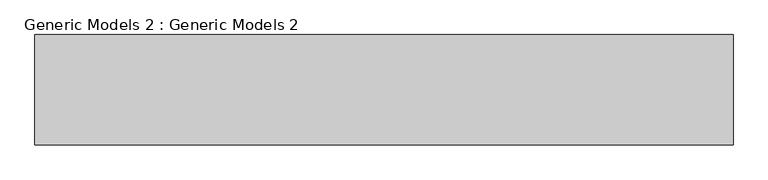
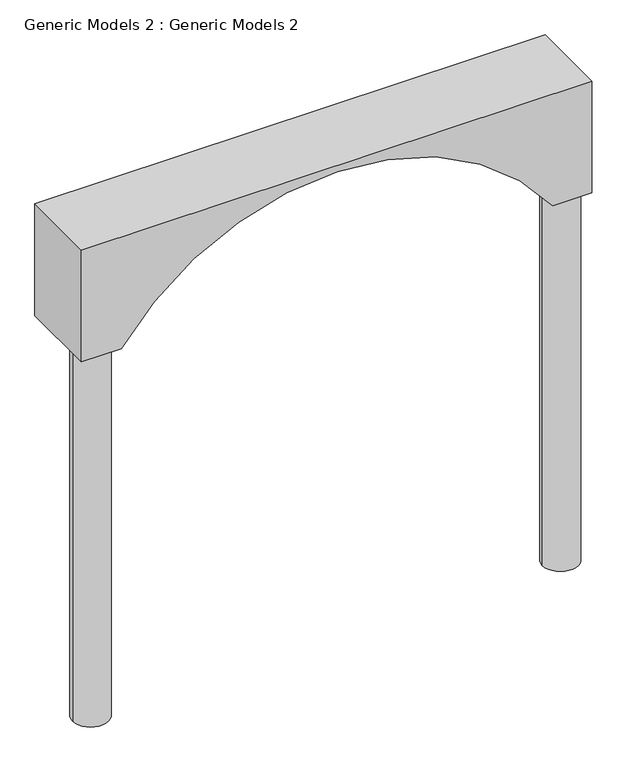
"""IFC4 building model written with IfcOpenShell, lengths in millimetres: proxy geometry, Generic Models 2 : Generic Models 2."""

from ifc_helpers import new_model, si_unit, point, frame, frame_2d, origin, origin_with_axes, place, context, project, spatial, polyline, circle_curve, trimmed, segment, composite_curve, outline, extrude, source, transform, mapped, element, save


def generic_models_2_generic_models_2_701112c8(model_context):
    return source(origin(), model_context, "Body", "SweptSolid", [
        extrude(outline(composite_curve([segment(trimmed(circle_curve(frame_2d((-14185.0310619, 3684.6465918)), 101.6), [point((-14286.6310619, 3684.6465918))], [point((-14083.4310619, 3684.6465918))], False, "CARTESIAN"), True, "CONTINUOUS"), segment(trimmed(circle_curve(frame_2d((-14185.0310619, 3684.6465918)), 101.6), [point((-14083.4310619, 3684.6465918))], [point((-14286.6310619, 3684.6465918))], False, "CARTESIAN"), True, "CONTINUOUS")], self_intersect=False)), origin_with_axes(), (0.0, 0.0, 1.0), 2226.4463041),
        extrude(outline(composite_curve([segment(trimmed(circle_curve(frame_2d((-11520.4016034, 3684.6465918)), 101.6), [point((-11418.8016034, 3684.6465918))], [point((-11622.0016034, 3684.6465918))], False, "CARTESIAN"), True, "CONTINUOUS"), segment(trimmed(circle_curve(frame_2d((-11520.4016034, 3684.6465918)), 101.6), [point((-11622.0016034, 3684.6465918))], [point((-11418.8016034, 3684.6465918))], False, "CARTESIAN"), True, "CONTINUOUS")], self_intersect=False)), origin_with_axes(), (0.0, 0.0, 1.0), 2226.4463041),
        extrude(outline(composite_curve([segment(polyline([(2226.4463041, -11627.5105536), (2226.4463041, -11405.0590017), (2895.6, -11405.0590017), (2895.6, -14300.3736637), (2226.4463041, -14300.3736637), (2226.4463041, -14074.0083114)]), True, "CONTINUOUS"), segment(trimmed(circle_curve(frame_2d((1360.7303343, -12850.7594325)), 1498.6), [point((2226.4463041, -14074.0083114))], [point((2226.4463041, -11627.5105536))], True, "CARTESIAN"), True, "CONTINUOUS")], self_intersect=False)), frame((0.0, 3574.2170165, 0.0), z_axis=(0.0, 1.0, 0.0), x_axis=(0.0, 0.0, 1.0)), (0.0, 0.0, 1.0), 457.2),
    ])


if __name__ == "__main__":
    model = new_model("IFC4")
    model_context = context("Model", 3, world=origin())
    ifc_project = project(units=[si_unit("LENGTHUNIT", "METRE", prefix="MILLI")], contexts=[model_context])
    site = spatial("IfcSite", under=ifc_project)
    building = spatial("IfcBuilding", under=site)
    placement = place(None, origin())
    generic_models_2_generic_models_2_shape = generic_models_2_generic_models_2_701112c8(model_context)
    element("IfcBuildingElementProxy", 1, Name="Generic Models 2 : Generic Models 2", ObjectType="Generic Models 2 : Generic Models 2", at=placement, inside=building, context=model_context, shape_type="MappedRepresentation", body=[
        mapped(generic_models_2_generic_models_2_shape, transform((0.0, 0.0, 0.0), x_axis=(1.0, 0.0, 0.0), y_axis=(0.0, 1.0, 0.0), z_axis=(0.0, 0.0, 1.0))),
    ])
    save(model, "model.ifc")
